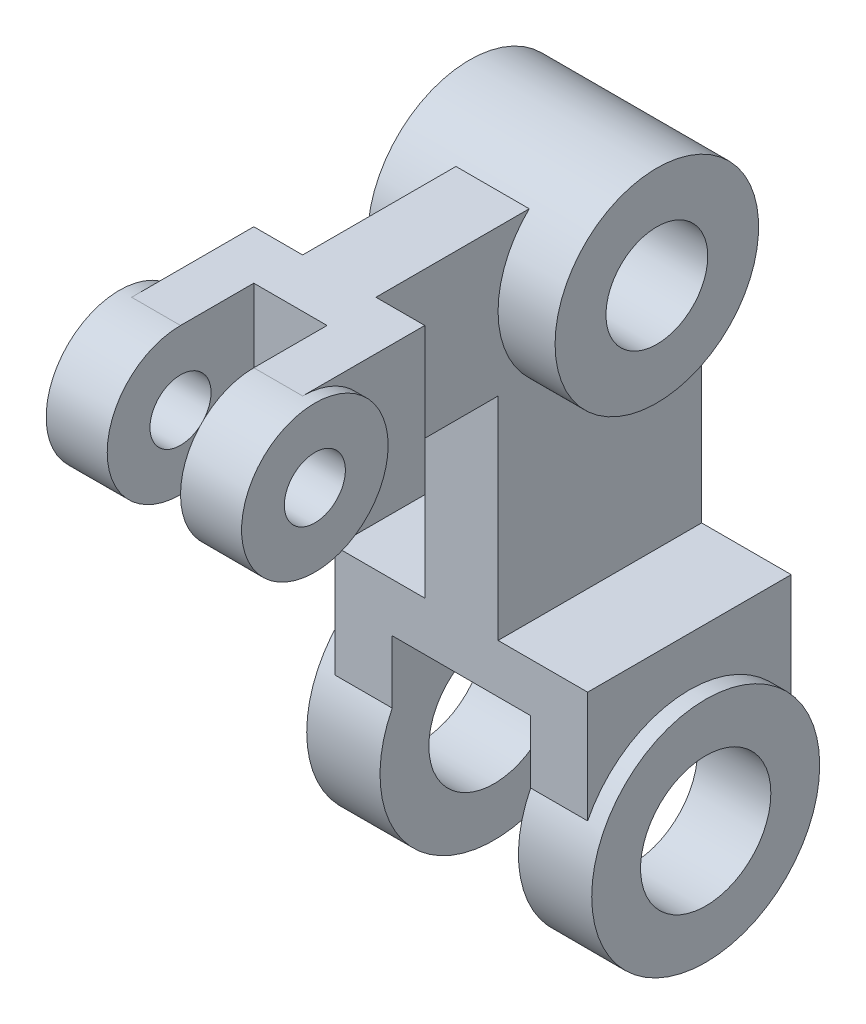
ISO-10303-21;
HEADER;
FILE_DESCRIPTION(('STEP AP214'),'2;1');
FILE_NAME('part.step','',(''),(''),'','','');
FILE_SCHEMA(('AUTOMOTIVE_DESIGN { 1 0 10303 214 1 1 1 1 }'));
ENDSEC;
DATA;
#1=APPLICATION_CONTEXT('core data for automotive mechanical design processes');
#2=APPLICATION_PROTOCOL_DEFINITION('international standard','automotive_design',2000,#1);
#3=PRODUCT_CONTEXT('',#1,'mechanical');
#4=PRODUCT('Part','Part','',(#3));
#5=PRODUCT_RELATED_PRODUCT_CATEGORY('part','',(#4));
#6=PRODUCT_DEFINITION_FORMATION('','',#4);
#7=PRODUCT_DEFINITION_CONTEXT('part definition',#1,'design');
#8=PRODUCT_DEFINITION('design','',#6,#7);
#9=PRODUCT_DEFINITION_SHAPE('','',#8);
#10=(LENGTH_UNIT() NAMED_UNIT(*) SI_UNIT(.MILLI.,.METRE.));
#11=(NAMED_UNIT(*) PLANE_ANGLE_UNIT() SI_UNIT($,.RADIAN.));
#12=(NAMED_UNIT(*) SI_UNIT($,.STERADIAN.) SOLID_ANGLE_UNIT());
#13=UNCERTAINTY_MEASURE_WITH_UNIT(LENGTH_MEASURE(1.E-05),#10,'distance_accuracy_value','');
#14=(GEOMETRIC_REPRESENTATION_CONTEXT(3) GLOBAL_UNCERTAINTY_ASSIGNED_CONTEXT((#13)) GLOBAL_UNIT_ASSIGNED_CONTEXT((#10,
#11,#12)) REPRESENTATION_CONTEXT('',''));
#15=CARTESIAN_POINT('',(0.,0.,0.));
#16=DIRECTION('',(0.,0.,1.));
#17=DIRECTION('',(1.,0.,0.));
#18=AXIS2_PLACEMENT_3D('',#15,#16,#17);
#19=CARTESIAN_POINT('',(-12.,110.,0.));
#20=DIRECTION('',(-1.,0.,0.));
#21=DIRECTION('',(0.,0.,1.));
#22=AXIS2_PLACEMENT_3D('',#19,#20,#21);
#23=CYLINDRICAL_SURFACE('',#22,25.);
#24=CARTESIAN_POINT('',(-12.,110.,0.));
#25=DIRECTION('',(-1.,0.,0.));
#26=DIRECTION('',(0.,0.,1.));
#27=AXIS2_PLACEMENT_3D('',#24,#25,#26);
#28=CIRCLE('',#27,25.);
#29=CARTESIAN_POINT('',(-12.,110.,25.));
#30=VERTEX_POINT('',#29);
#31=EDGE_CURVE('E265',#30,#30,#28,.T.);
#32=ORIENTED_EDGE('',*,*,#31,.T.);
#33=EDGE_LOOP('',(#32));
#34=FACE_BOUND('',#33,.T.);
#35=CARTESIAN_POINT('',(-58.,110.,0.));
#36=DIRECTION('',(-1.,0.,0.));
#37=DIRECTION('',(0.,0.,1.));
#38=AXIS2_PLACEMENT_3D('',#35,#36,#37);
#39=CIRCLE('',#38,25.);
#40=CARTESIAN_POINT('',(-58.,110.,25.));
#41=VERTEX_POINT('',#40);
#42=EDGE_CURVE('E258',#41,#41,#39,.T.);
#43=ORIENTED_EDGE('',*,*,#42,.F.);
#44=EDGE_LOOP('',(#43));
#45=FACE_BOUND('',#44,.T.);
#46=DIRECTION('',(-1.,0.,0.));
#47=VECTOR('',#46,1.);
#48=CARTESIAN_POINT('',(-12.,128.,17.3493515728975));
#49=LINE('',#48,#47);
#50=CARTESIAN_POINT('',(-44.,128.,17.3493515728975));
#51=VERTEX_POINT('',#50);
#52=CARTESIAN_POINT('',(-26.,128.,17.3493515728975));
#53=VERTEX_POINT('',#52);
#54=EDGE_CURVE('E11',#51,#53,#49,.F.);
#55=ORIENTED_EDGE('',*,*,#54,.T.);
#56=CARTESIAN_POINT('',(-26.,110.,0.));
#57=DIRECTION('',(1.,0.,0.));
#58=DIRECTION('',(0.,1.,0.));
#59=AXIS2_PLACEMENT_3D('',#56,#57,#58);
#60=CIRCLE('',#59,25.);
#61=CARTESIAN_POINT('',(-26.,110.,-25.));
#62=VERTEX_POINT('',#61);
#63=EDGE_CURVE('E57',#53,#62,#60,.T.);
#64=ORIENTED_EDGE('',*,*,#63,.T.);
#65=DIRECTION('',(-1.,0.,0.));
#66=VECTOR('',#65,1.);
#67=CARTESIAN_POINT('',(-44.,110.,-25.));
#68=LINE('',#67,#66);
#69=CARTESIAN_POINT('',(-44.,110.,-25.));
#70=VERTEX_POINT('',#69);
#71=EDGE_CURVE('E275',#62,#70,#68,.T.);
#72=ORIENTED_EDGE('',*,*,#71,.T.);
#73=CARTESIAN_POINT('',(-44.,110.,0.));
#74=DIRECTION('',(-1.,0.,0.));
#75=DIRECTION('',(0.,0.,1.));
#76=AXIS2_PLACEMENT_3D('',#73,#74,#75);
#77=CIRCLE('',#76,25.);
#78=EDGE_CURVE('E261',#70,#51,#77,.T.);
#79=ORIENTED_EDGE('',*,*,#78,.T.);
#80=EDGE_LOOP('',(#55,#64,#72,#79));
#81=FACE_BOUND('',#80,.T.);
#82=ADVANCED_FACE('F50',(#34,#45,#81),#23,.T.);
#83=CARTESIAN_POINT('',(0.,40.,28.));
#84=DIRECTION('',(0.,-1.,0.));
#85=DIRECTION('',(1.,0.,0.));
#86=AXIS2_PLACEMENT_3D('',#83,#84,#85);
#87=PLANE('',#86);
#88=DIRECTION('',(0.,0.,1.));
#89=VECTOR('',#88,1.);
#90=CARTESIAN_POINT('',(-44.,40.,-25.));
#91=LINE('',#90,#89);
#92=CARTESIAN_POINT('',(-44.,40.,-25.));
#93=VERTEX_POINT('',#92);
#94=CARTESIAN_POINT('',(-44.,40.,25.));
#95=VERTEX_POINT('',#94);
#96=EDGE_CURVE('E273',#93,#95,#91,.T.);
#97=ORIENTED_EDGE('',*,*,#96,.F.);
#98=DIRECTION('',(1.,0.,0.));
#99=VECTOR('',#98,1.);
#100=CARTESIAN_POINT('',(-78.,40.,-25.));
#101=LINE('',#100,#99);
#102=CARTESIAN_POINT('',(-66.,40.,-25.));
#103=VERTEX_POINT('',#102);
#104=EDGE_CURVE('E297',#103,#93,#101,.T.);
#105=ORIENTED_EDGE('',*,*,#104,.F.);
#106=DIRECTION('',(0.,0.,-1.));
#107=VECTOR('',#106,1.);
#108=CARTESIAN_POINT('',(-66.,40.,28.));
#109=LINE('',#108,#107);
#110=CARTESIAN_POINT('',(-66.,40.,25.));
#111=VERTEX_POINT('',#110);
#112=EDGE_CURVE('E347',#111,#103,#109,.T.);
#113=ORIENTED_EDGE('',*,*,#112,.F.);
#114=DIRECTION('',(1.,0.,0.));
#115=VECTOR('',#114,1.);
#116=CARTESIAN_POINT('',(-78.,40.,25.));
#117=LINE('',#116,#115);
#118=EDGE_CURVE('E289',#111,#95,#117,.T.);
#119=ORIENTED_EDGE('',*,*,#118,.T.);
#120=EDGE_LOOP('',(#97,#105,#113,#119));
#121=FACE_BOUND('',#120,.T.);
#122=ADVANCED_FACE('F476',(#121),#87,.F.);
#123=CARTESIAN_POINT('',(-70.,0.,0.));
#124=DIRECTION('',(1.,0.,0.));
#125=DIRECTION('',(0.,0.,-1.));
#126=AXIS2_PLACEMENT_3D('',#123,#124,#125);
#127=CYLINDRICAL_SURFACE('',#126,28.);
#128=DIRECTION('',(1.,0.,0.));
#129=VECTOR('',#128,1.);
#130=CARTESIAN_POINT('',(-78.,12.6095202129185,25.));
#131=LINE('',#130,#129);
#132=CARTESIAN_POINT('',(-66.,12.6095202129185,25.));
#133=VERTEX_POINT('',#132);
#134=CARTESIAN_POINT('',(-52.,12.6095202129185,25.));
#135=VERTEX_POINT('',#134);
#136=EDGE_CURVE('E295',#133,#135,#131,.T.);
#137=ORIENTED_EDGE('',*,*,#136,.F.);
#138=CARTESIAN_POINT('',(-66.,0.,0.));
#139=DIRECTION('',(1.,0.,0.));
#140=DIRECTION('',(0.,0.,-1.));
#141=AXIS2_PLACEMENT_3D('',#138,#139,#140);
#142=CIRCLE('',#141,28.);
#143=CARTESIAN_POINT('',(-66.,12.6095202129185,-25.));
#144=VERTEX_POINT('',#143);
#145=EDGE_CURVE('E333',#133,#144,#142,.F.);
#146=ORIENTED_EDGE('',*,*,#145,.T.);
#147=DIRECTION('',(1.,0.,0.));
#148=VECTOR('',#147,1.);
#149=CARTESIAN_POINT('',(-78.,12.6095202129185,-25.));
#150=LINE('',#149,#148);
#151=CARTESIAN_POINT('',(-52.,12.6095202129185,-25.));
#152=VERTEX_POINT('',#151);
#153=EDGE_CURVE('E287',#144,#152,#150,.T.);
#154=ORIENTED_EDGE('',*,*,#153,.T.);
#155=CARTESIAN_POINT('',(-52.,0.,0.));
#156=DIRECTION('',(-1.,0.,0.));
#157=DIRECTION('',(0.,0.,1.));
#158=AXIS2_PLACEMENT_3D('',#155,#156,#157);
#159=CIRCLE('',#158,28.);
#160=EDGE_CURVE('E326',#152,#135,#159,.T.);
#161=ORIENTED_EDGE('',*,*,#160,.T.);
#162=EDGE_LOOP('',(#137,#146,#154,#161));
#163=FACE_BOUND('',#162,.T.);
#164=CARTESIAN_POINT('',(-70.,0.,0.));
#165=DIRECTION('',(-1.,0.,0.));
#166=DIRECTION('',(0.,0.,1.));
#167=AXIS2_PLACEMENT_3D('',#164,#165,#166);
#168=CIRCLE('',#167,28.);
#169=CARTESIAN_POINT('',(-70.,0.,28.));
#170=VERTEX_POINT('',#169);
#171=EDGE_CURVE('E331',#170,#170,#168,.T.);
#172=ORIENTED_EDGE('',*,*,#171,.F.);
#173=EDGE_LOOP('',(#172));
#174=FACE_BOUND('',#173,.T.);
#175=ADVANCED_FACE('F487',(#163,#174),#127,.T.);
#176=CARTESIAN_POINT('',(-18.,0.,0.));
#177=DIRECTION('',(1.,0.,0.));
#178=DIRECTION('',(0.,0.,-1.));
#179=AXIS2_PLACEMENT_3D('',#176,#177,#178);
#180=CYLINDRICAL_SURFACE('',#179,28.);
#181=CARTESIAN_POINT('',(-4.,0.,0.));
#182=DIRECTION('',(1.,0.,0.));
#183=DIRECTION('',(0.,0.,-1.));
#184=AXIS2_PLACEMENT_3D('',#181,#182,#183);
#185=CIRCLE('',#184,28.);
#186=CARTESIAN_POINT('',(-4.,12.6095202129185,25.));
#187=VERTEX_POINT('',#186);
#188=CARTESIAN_POINT('',(-4.,12.6095202129185,-25.));
#189=VERTEX_POINT('',#188);
#190=EDGE_CURVE('E352',#187,#189,#185,.F.);
#191=ORIENTED_EDGE('',*,*,#190,.F.);
#192=CARTESIAN_POINT('',(-18.,12.6095202129185,25.));
#193=VERTEX_POINT('',#192);
#194=EDGE_CURVE('E286',#193,#187,#131,.T.);
#195=ORIENTED_EDGE('',*,*,#194,.F.);
#196=CARTESIAN_POINT('',(-18.,0.,0.));
#197=DIRECTION('',(1.,0.,0.));
#198=DIRECTION('',(0.,0.,-1.));
#199=AXIS2_PLACEMENT_3D('',#196,#197,#198);
#200=CIRCLE('',#199,28.);
#201=CARTESIAN_POINT('',(-18.,12.6095202129185,-25.));
#202=VERTEX_POINT('',#201);
#203=EDGE_CURVE('E365',#193,#202,#200,.T.);
#204=ORIENTED_EDGE('',*,*,#203,.T.);
#205=EDGE_CURVE('E296',#202,#189,#150,.T.);
#206=ORIENTED_EDGE('',*,*,#205,.T.);
#207=EDGE_LOOP('',(#191,#195,#204,#206));
#208=FACE_BOUND('',#207,.T.);
#209=CARTESIAN_POINT('',(0.,0.,0.));
#210=DIRECTION('',(1.,0.,0.));
#211=DIRECTION('',(0.,0.,-1.));
#212=AXIS2_PLACEMENT_3D('',#209,#210,#211);
#213=CIRCLE('',#212,28.);
#214=CARTESIAN_POINT('',(0.,0.,-28.));
#215=VERTEX_POINT('',#214);
#216=EDGE_CURVE('E363',#215,#215,#213,.T.);
#217=ORIENTED_EDGE('',*,*,#216,.F.);
#218=EDGE_LOOP('',(#217));
#219=FACE_BOUND('',#218,.T.);
#220=ADVANCED_FACE('F47',(#208,#219),#180,.T.);
#221=CARTESIAN_POINT('',(-66.,0.,28.));
#222=DIRECTION('',(1.,0.,0.));
#223=DIRECTION('',(0.,0.,-1.));
#224=AXIS2_PLACEMENT_3D('',#221,#222,#223);
#225=PLANE('',#224);
#226=ORIENTED_EDGE('',*,*,#145,.F.);
#227=DIRECTION('',(0.,1.,0.));
#228=VECTOR('',#227,1.);
#229=CARTESIAN_POINT('',(-66.,0.,25.));
#230=LINE('',#229,#228);
#231=EDGE_CURVE('E325',#133,#111,#230,.T.);
#232=ORIENTED_EDGE('',*,*,#231,.T.);
#233=ORIENTED_EDGE('',*,*,#112,.T.);
#234=DIRECTION('',(0.,-1.,0.));
#235=VECTOR('',#234,1.);
#236=CARTESIAN_POINT('',(-66.,0.,-25.));
#237=LINE('',#236,#235);
#238=EDGE_CURVE('E311',#103,#144,#237,.T.);
#239=ORIENTED_EDGE('',*,*,#238,.T.);
#240=EDGE_LOOP('',(#226,#232,#233,#239));
#241=FACE_BOUND('',#240,.T.);
#242=ADVANCED_FACE('F484',(#241),#225,.F.);
#243=CARTESIAN_POINT('',(-18.,0.,0.));
#244=DIRECTION('',(1.,0.,0.));
#245=DIRECTION('',(0.,0.,-1.));
#246=AXIS2_PLACEMENT_3D('',#243,#244,#245);
#247=PLANE('',#246);
#248=ORIENTED_EDGE('',*,*,#203,.F.);
#249=DIRECTION('',(0.,1.,0.));
#250=VECTOR('',#249,1.);
#251=CARTESIAN_POINT('',(-18.,0.,25.));
#252=LINE('',#251,#250);
#253=CARTESIAN_POINT('',(-18.,28.,25.));
#254=VERTEX_POINT('',#253);
#255=EDGE_CURVE('E318',#193,#254,#252,.T.);
#256=ORIENTED_EDGE('',*,*,#255,.T.);
#257=DIRECTION('',(0.,0.,-1.));
#258=VECTOR('',#257,1.);
#259=CARTESIAN_POINT('',(-18.,28.,28.));
#260=LINE('',#259,#258);
#261=CARTESIAN_POINT('',(-18.,28.,-25.));
#262=VERTEX_POINT('',#261);
#263=EDGE_CURVE('E338',#254,#262,#260,.T.);
#264=ORIENTED_EDGE('',*,*,#263,.T.);
#265=DIRECTION('',(0.,-1.,0.));
#266=VECTOR('',#265,1.);
#267=CARTESIAN_POINT('',(-18.,0.,-25.));
#268=LINE('',#267,#266);
#269=EDGE_CURVE('E308',#262,#202,#268,.T.);
#270=ORIENTED_EDGE('',*,*,#269,.T.);
#271=EDGE_LOOP('',(#248,#256,#264,#270));
#272=FACE_BOUND('',#271,.T.);
#273=CARTESIAN_POINT('',(-18.,0.,0.));
#274=DIRECTION('',(1.,0.,0.));
#275=DIRECTION('',(0.,0.,-1.));
#276=AXIS2_PLACEMENT_3D('',#273,#274,#275);
#277=CIRCLE('',#276,16.);
#278=CARTESIAN_POINT('',(-18.,0.,-16.));
#279=VERTEX_POINT('',#278);
#280=EDGE_CURVE('E356',#279,#279,#277,.T.);
#281=ORIENTED_EDGE('',*,*,#280,.T.);
#282=EDGE_LOOP('',(#281));
#283=FACE_BOUND('',#282,.T.);
#284=ADVANCED_FACE('F502',(#272,#283),#247,.F.);
#285=CARTESIAN_POINT('',(0.,0.,0.));
#286=DIRECTION('',(1.,0.,0.));
#287=DIRECTION('',(0.,0.,-1.));
#288=AXIS2_PLACEMENT_3D('',#285,#286,#287);
#289=PLANE('',#288);
#290=CARTESIAN_POINT('',(0.,0.,0.));
#291=DIRECTION('',(1.,0.,0.));
#292=DIRECTION('',(0.,0.,-1.));
#293=AXIS2_PLACEMENT_3D('',#290,#291,#292);
#294=CIRCLE('',#293,16.);
#295=CARTESIAN_POINT('',(0.,0.,-16.));
#296=VERTEX_POINT('',#295);
#297=EDGE_CURVE('E355',#296,#296,#294,.T.);
#298=ORIENTED_EDGE('',*,*,#297,.F.);
#299=EDGE_LOOP('',(#298));
#300=FACE_BOUND('',#299,.T.);
#301=ORIENTED_EDGE('',*,*,#216,.T.);
#302=EDGE_LOOP('',(#301));
#303=FACE_BOUND('',#302,.T.);
#304=ADVANCED_FACE('F520',(#300,#303),#289,.T.);
#305=CARTESIAN_POINT('',(-95.,0.,0.));
#306=DIRECTION('',(1.,0.,0.));
#307=DIRECTION('',(0.,0.,-1.));
#308=AXIS2_PLACEMENT_3D('',#305,#306,#307);
#309=CYLINDRICAL_SURFACE('',#308,16.);
#310=ORIENTED_EDGE('',*,*,#280,.F.);
#311=EDGE_LOOP('',(#310));
#312=FACE_BOUND('',#311,.T.);
#313=ORIENTED_EDGE('',*,*,#297,.T.);
#314=EDGE_LOOP('',(#313));
#315=FACE_BOUND('',#314,.T.);
#316=ADVANCED_FACE('F517',(#312,#315),#309,.F.);
#317=CARTESIAN_POINT('',(-4.,0.,28.));
#318=DIRECTION('',(1.,0.,0.));
#319=DIRECTION('',(0.,0.,-1.));
#320=AXIS2_PLACEMENT_3D('',#317,#318,#319);
#321=PLANE('',#320);
#322=DIRECTION('',(0.,1.,0.));
#323=VECTOR('',#322,1.);
#324=CARTESIAN_POINT('',(-4.,0.,25.));
#325=LINE('',#324,#323);
#326=CARTESIAN_POINT('',(-4.,40.,25.));
#327=VERTEX_POINT('',#326);
#328=EDGE_CURVE('E283',#187,#327,#325,.T.);
#329=ORIENTED_EDGE('',*,*,#328,.F.);
#330=ORIENTED_EDGE('',*,*,#190,.T.);
#331=DIRECTION('',(0.,-1.,0.));
#332=VECTOR('',#331,1.);
#333=CARTESIAN_POINT('',(-4.,0.,-25.));
#334=LINE('',#333,#332);
#335=CARTESIAN_POINT('',(-4.,40.,-25.));
#336=VERTEX_POINT('',#335);
#337=EDGE_CURVE('E277',#336,#189,#334,.T.);
#338=ORIENTED_EDGE('',*,*,#337,.F.);
#339=DIRECTION('',(0.,0.,-1.));
#340=VECTOR('',#339,1.);
#341=CARTESIAN_POINT('',(-4.,40.,28.));
#342=LINE('',#341,#340);
#343=EDGE_CURVE('E349',#327,#336,#342,.T.);
#344=ORIENTED_EDGE('',*,*,#343,.F.);
#345=EDGE_LOOP('',(#329,#330,#338,#344));
#346=FACE_BOUND('',#345,.T.);
#347=ADVANCED_FACE('F499',(#346),#321,.T.);
#348=CARTESIAN_POINT('',(-26.,40.,-25.));
#349=VERTEX_POINT('',#348);
#350=EDGE_CURVE('E300',#349,#336,#101,.T.);
#351=ORIENTED_EDGE('',*,*,#350,.F.);
#352=DIRECTION('',(0.,0.,1.));
#353=VECTOR('',#352,1.);
#354=CARTESIAN_POINT('',(-26.,40.,-25.));
#355=LINE('',#354,#353);
#356=CARTESIAN_POINT('',(-26.,40.,25.));
#357=VERTEX_POINT('',#356);
#358=EDGE_CURVE('E280',#349,#357,#355,.T.);
#359=ORIENTED_EDGE('',*,*,#358,.T.);
#360=EDGE_CURVE('E292',#357,#327,#117,.T.);
#361=ORIENTED_EDGE('',*,*,#360,.T.);
#362=ORIENTED_EDGE('',*,*,#343,.T.);
#363=EDGE_LOOP('',(#351,#359,#361,#362));
#364=FACE_BOUND('',#363,.T.);
#365=ADVANCED_FACE('F495',(#364),#87,.F.);
#366=CARTESIAN_POINT('',(-52.,0.,28.));
#367=DIRECTION('',(-1.,0.,0.));
#368=DIRECTION('',(0.,0.,1.));
#369=AXIS2_PLACEMENT_3D('',#366,#367,#368);
#370=PLANE('',#369);
#371=DIRECTION('',(0.,-1.,0.));
#372=VECTOR('',#371,1.);
#373=CARTESIAN_POINT('',(-52.,0.,25.));
#374=LINE('',#373,#372);
#375=CARTESIAN_POINT('',(-52.,28.,25.));
#376=VERTEX_POINT('',#375);
#377=EDGE_CURVE('E320',#376,#135,#374,.T.);
#378=ORIENTED_EDGE('',*,*,#377,.T.);
#379=ORIENTED_EDGE('',*,*,#160,.F.);
#380=DIRECTION('',(0.,1.,0.));
#381=VECTOR('',#380,1.);
#382=CARTESIAN_POINT('',(-52.,0.,-25.));
#383=LINE('',#382,#381);
#384=CARTESIAN_POINT('',(-52.,28.,-25.));
#385=VERTEX_POINT('',#384);
#386=EDGE_CURVE('E304',#152,#385,#383,.T.);
#387=ORIENTED_EDGE('',*,*,#386,.T.);
#388=DIRECTION('',(0.,0.,-1.));
#389=VECTOR('',#388,1.);
#390=CARTESIAN_POINT('',(-52.,28.,28.));
#391=LINE('',#390,#389);
#392=EDGE_CURVE('E345',#376,#385,#391,.T.);
#393=ORIENTED_EDGE('',*,*,#392,.F.);
#394=EDGE_LOOP('',(#378,#379,#387,#393));
#395=FACE_BOUND('',#394,.T.);
#396=CARTESIAN_POINT('',(-52.,0.,0.));
#397=DIRECTION('',(-1.,0.,0.));
#398=DIRECTION('',(0.,0.,1.));
#399=AXIS2_PLACEMENT_3D('',#396,#397,#398);
#400=CIRCLE('',#399,16.);
#401=CARTESIAN_POINT('',(-52.,0.,16.));
#402=VERTEX_POINT('',#401);
#403=EDGE_CURVE('E327',#402,#402,#400,.T.);
#404=ORIENTED_EDGE('',*,*,#403,.T.);
#405=EDGE_LOOP('',(#404));
#406=FACE_BOUND('',#405,.T.);
#407=ADVANCED_FACE('F515',(#395,#406),#370,.F.);
#408=CARTESIAN_POINT('',(0.,28.,28.));
#409=DIRECTION('',(0.,1.,0.));
#410=DIRECTION('',(0.,0.,1.));
#411=AXIS2_PLACEMENT_3D('',#408,#409,#410);
#412=PLANE('',#411);
#413=ORIENTED_EDGE('',*,*,#263,.F.);
#414=DIRECTION('',(-1.,0.,0.));
#415=VECTOR('',#414,1.);
#416=CARTESIAN_POINT('',(0.,28.,25.));
#417=LINE('',#416,#415);
#418=EDGE_CURVE('E313',#254,#376,#417,.T.);
#419=ORIENTED_EDGE('',*,*,#418,.T.);
#420=ORIENTED_EDGE('',*,*,#392,.T.);
#421=DIRECTION('',(1.,0.,0.));
#422=VECTOR('',#421,1.);
#423=CARTESIAN_POINT('',(0.,28.,-25.));
#424=LINE('',#423,#422);
#425=EDGE_CURVE('E293',#385,#262,#424,.T.);
#426=ORIENTED_EDGE('',*,*,#425,.T.);
#427=EDGE_LOOP('',(#413,#419,#420,#426));
#428=FACE_BOUND('',#427,.T.);
#429=ADVANCED_FACE('F507',(#428),#412,.F.);
#430=CARTESIAN_POINT('',(-70.,0.,0.));
#431=DIRECTION('',(-1.,0.,0.));
#432=DIRECTION('',(0.,0.,1.));
#433=AXIS2_PLACEMENT_3D('',#430,#431,#432);
#434=PLANE('',#433);
#435=CARTESIAN_POINT('',(-70.,0.,0.));
#436=DIRECTION('',(-1.,0.,0.));
#437=DIRECTION('',(0.,0.,1.));
#438=AXIS2_PLACEMENT_3D('',#435,#436,#437);
#439=CIRCLE('',#438,16.);
#440=CARTESIAN_POINT('',(-70.,0.,16.));
#441=VERTEX_POINT('',#440);
#442=EDGE_CURVE('E330',#441,#441,#439,.T.);
#443=ORIENTED_EDGE('',*,*,#442,.F.);
#444=EDGE_LOOP('',(#443));
#445=FACE_BOUND('',#444,.T.);
#446=ORIENTED_EDGE('',*,*,#171,.T.);
#447=EDGE_LOOP('',(#446));
#448=FACE_BOUND('',#447,.T.);
#449=ADVANCED_FACE('F551',(#445,#448),#434,.T.);
#450=CARTESIAN_POINT('',(-95.,0.,0.));
#451=DIRECTION('',(1.,0.,0.));
#452=DIRECTION('',(0.,0.,-1.));
#453=AXIS2_PLACEMENT_3D('',#450,#451,#452);
#454=CYLINDRICAL_SURFACE('',#453,16.);
#455=ORIENTED_EDGE('',*,*,#403,.F.);
#456=EDGE_LOOP('',(#455));
#457=FACE_BOUND('',#456,.T.);
#458=ORIENTED_EDGE('',*,*,#442,.T.);
#459=EDGE_LOOP('',(#458));
#460=FACE_BOUND('',#459,.T.);
#461=ADVANCED_FACE('F550',(#457,#460),#454,.F.);
#462=CARTESIAN_POINT('',(-78.,0.,-25.));
#463=DIRECTION('',(0.,0.,1.));
#464=DIRECTION('',(0.,-1.,0.));
#465=AXIS2_PLACEMENT_3D('',#462,#463,#464);
#466=PLANE('',#465);
#467=ORIENTED_EDGE('',*,*,#104,.T.);
#468=DIRECTION('',(0.,-1.,0.));
#469=VECTOR('',#468,1.);
#470=CARTESIAN_POINT('',(-44.,40.,-25.));
#471=LINE('',#470,#469);
#472=EDGE_CURVE('E269',#70,#93,#471,.T.);
#473=ORIENTED_EDGE('',*,*,#472,.F.);
#474=ORIENTED_EDGE('',*,*,#71,.F.);
#475=DIRECTION('',(0.,1.,0.));
#476=VECTOR('',#475,1.);
#477=CARTESIAN_POINT('',(-26.,110.,-25.));
#478=LINE('',#477,#476);
#479=EDGE_CURVE('E270',#349,#62,#478,.T.);
#480=ORIENTED_EDGE('',*,*,#479,.F.);
#481=ORIENTED_EDGE('',*,*,#350,.T.);
#482=ORIENTED_EDGE('',*,*,#337,.T.);
#483=ORIENTED_EDGE('',*,*,#205,.F.);
#484=ORIENTED_EDGE('',*,*,#269,.F.);
#485=ORIENTED_EDGE('',*,*,#425,.F.);
#486=ORIENTED_EDGE('',*,*,#386,.F.);
#487=ORIENTED_EDGE('',*,*,#153,.F.);
#488=ORIENTED_EDGE('',*,*,#238,.F.);
#489=EDGE_LOOP('',(#467,#473,#474,#480,#481,#482,#483,#484,#485,#486,#487,#488));
#490=FACE_BOUND('',#489,.T.);
#491=ADVANCED_FACE('F472',(#490),#466,.F.);
#492=CARTESIAN_POINT('',(-78.,0.,25.));
#493=DIRECTION('',(0.,0.,-1.));
#494=DIRECTION('',(-1.,0.,0.));
#495=AXIS2_PLACEMENT_3D('',#492,#493,#494);
#496=PLANE('',#495);
#497=DIRECTION('',(0.,1.,0.));
#498=VECTOR('',#497,1.);
#499=CARTESIAN_POINT('',(-26.,110.,25.));
#500=LINE('',#499,#498);
#501=CARTESIAN_POINT('',(-26.,92.,25.));
#502=VERTEX_POINT('',#501);
#503=EDGE_CURVE('E66',#357,#502,#500,.T.);
#504=ORIENTED_EDGE('',*,*,#503,.T.);
#505=DIRECTION('',(-1.,0.,0.));
#506=VECTOR('',#505,1.);
#507=CARTESIAN_POINT('',(-78.,92.,25.));
#508=LINE('',#507,#506);
#509=CARTESIAN_POINT('',(-44.,92.,25.));
#510=VERTEX_POINT('',#509);
#511=EDGE_CURVE('E259',#502,#510,#508,.T.);
#512=ORIENTED_EDGE('',*,*,#511,.T.);
#513=DIRECTION('',(0.,-1.,0.));
#514=VECTOR('',#513,1.);
#515=CARTESIAN_POINT('',(-44.,40.,25.));
#516=LINE('',#515,#514);
#517=EDGE_CURVE('E267',#510,#95,#516,.T.);
#518=ORIENTED_EDGE('',*,*,#517,.T.);
#519=ORIENTED_EDGE('',*,*,#118,.F.);
#520=ORIENTED_EDGE('',*,*,#231,.F.);
#521=ORIENTED_EDGE('',*,*,#136,.T.);
#522=ORIENTED_EDGE('',*,*,#377,.F.);
#523=ORIENTED_EDGE('',*,*,#418,.F.);
#524=ORIENTED_EDGE('',*,*,#255,.F.);
#525=ORIENTED_EDGE('',*,*,#194,.T.);
#526=ORIENTED_EDGE('',*,*,#328,.T.);
#527=ORIENTED_EDGE('',*,*,#360,.F.);
#528=EDGE_LOOP('',(#504,#512,#518,#519,#520,#521,#522,#523,#524,#525,#526,#527));
#529=FACE_BOUND('',#528,.T.);
#530=ADVANCED_FACE('F442',(#529),#496,.F.);
#531=CARTESIAN_POINT('',(-44.,40.,-25.));
#532=DIRECTION('',(-1.,0.,0.));
#533=DIRECTION('',(0.,0.,1.));
#534=AXIS2_PLACEMENT_3D('',#531,#532,#533);
#535=PLANE('',#534);
#536=ORIENTED_EDGE('',*,*,#517,.F.);
#537=DIRECTION('',(0.,0.,1.));
#538=VECTOR('',#537,1.);
#539=CARTESIAN_POINT('',(-44.,92.,55.));
#540=LINE('',#539,#538);
#541=CARTESIAN_POINT('',(-44.,92.,55.));
#542=VERTEX_POINT('',#541);
#543=EDGE_CURVE('E424',#510,#542,#540,.T.);
#544=ORIENTED_EDGE('',*,*,#543,.T.);
#545=DIRECTION('',(0.,-1.,0.));
#546=VECTOR('',#545,1.);
#547=CARTESIAN_POINT('',(-44.,128.,55.));
#548=LINE('',#547,#546);
#549=CARTESIAN_POINT('',(-44.,128.,55.));
#550=VERTEX_POINT('',#549);
#551=EDGE_CURVE('E250',#550,#542,#548,.T.);
#552=ORIENTED_EDGE('',*,*,#551,.F.);
#553=DIRECTION('',(0.,0.,1.));
#554=VECTOR('',#553,1.);
#555=CARTESIAN_POINT('',(-44.,128.,55.));
#556=LINE('',#555,#554);
#557=EDGE_CURVE('E404',#51,#550,#556,.T.);
#558=ORIENTED_EDGE('',*,*,#557,.F.);
#559=ORIENTED_EDGE('',*,*,#78,.F.);
#560=ORIENTED_EDGE('',*,*,#472,.T.);
#561=ORIENTED_EDGE('',*,*,#96,.T.);
#562=EDGE_LOOP('',(#536,#544,#552,#558,#559,#560,#561));
#563=FACE_BOUND('',#562,.T.);
#564=ADVANCED_FACE('F439',(#563),#535,.T.);
#565=CARTESIAN_POINT('',(-26.,110.,-25.));
#566=DIRECTION('',(1.,0.,0.));
#567=DIRECTION('',(0.,1.,0.));
#568=AXIS2_PLACEMENT_3D('',#565,#566,#567);
#569=PLANE('',#568);
#570=ORIENTED_EDGE('',*,*,#479,.T.);
#571=ORIENTED_EDGE('',*,*,#63,.F.);
#572=DIRECTION('',(0.,0.,-1.));
#573=VECTOR('',#572,1.);
#574=CARTESIAN_POINT('',(-26.,128.,0.));
#575=LINE('',#574,#573);
#576=CARTESIAN_POINT('',(-26.,128.,55.));
#577=VERTEX_POINT('',#576);
#578=EDGE_CURVE('E405',#577,#53,#575,.T.);
#579=ORIENTED_EDGE('',*,*,#578,.F.);
#580=DIRECTION('',(0.,-1.,0.));
#581=VECTOR('',#580,1.);
#582=CARTESIAN_POINT('',(-26.,128.,55.));
#583=LINE('',#582,#581);
#584=CARTESIAN_POINT('',(-26.,92.,55.));
#585=VERTEX_POINT('',#584);
#586=EDGE_CURVE('E249',#577,#585,#583,.T.);
#587=ORIENTED_EDGE('',*,*,#586,.T.);
#588=DIRECTION('',(0.,0.,-1.));
#589=VECTOR('',#588,1.);
#590=CARTESIAN_POINT('',(-26.,92.,0.));
#591=LINE('',#590,#589);
#592=EDGE_CURVE('E421',#585,#502,#591,.T.);
#593=ORIENTED_EDGE('',*,*,#592,.T.);
#594=ORIENTED_EDGE('',*,*,#503,.F.);
#595=ORIENTED_EDGE('',*,*,#358,.F.);
#596=EDGE_LOOP('',(#570,#571,#579,#587,#593,#594,#595));
#597=FACE_BOUND('',#596,.T.);
#598=ADVANCED_FACE('F450',(#597),#569,.T.);
#599=CARTESIAN_POINT('',(-12.,110.,0.));
#600=DIRECTION('',(-1.,0.,0.));
#601=DIRECTION('',(0.,0.,1.));
#602=AXIS2_PLACEMENT_3D('',#599,#600,#601);
#603=PLANE('',#602);
#604=CARTESIAN_POINT('',(-12.,110.,0.));
#605=DIRECTION('',(1.,0.,0.));
#606=DIRECTION('',(0.,0.,-1.));
#607=AXIS2_PLACEMENT_3D('',#604,#605,#606);
#608=CIRCLE('',#607,12.5);
#609=CARTESIAN_POINT('',(-12.,110.,-12.5));
#610=VERTEX_POINT('',#609);
#611=EDGE_CURVE('E378',#610,#610,#608,.T.);
#612=ORIENTED_EDGE('',*,*,#611,.F.);
#613=EDGE_LOOP('',(#612));
#614=FACE_BOUND('',#613,.T.);
#615=ORIENTED_EDGE('',*,*,#31,.F.);
#616=EDGE_LOOP('',(#615));
#617=FACE_BOUND('',#616,.T.);
#618=ADVANCED_FACE('F537',(#614,#617),#603,.F.);
#619=CARTESIAN_POINT('',(-58.,110.,0.));
#620=DIRECTION('',(-1.,0.,0.));
#621=DIRECTION('',(0.,0.,1.));
#622=AXIS2_PLACEMENT_3D('',#619,#620,#621);
#623=PLANE('',#622);
#624=CARTESIAN_POINT('',(-58.,110.,0.));
#625=DIRECTION('',(-1.,0.,0.));
#626=DIRECTION('',(0.,0.,1.));
#627=AXIS2_PLACEMENT_3D('',#624,#625,#626);
#628=CIRCLE('',#627,12.5);
#629=CARTESIAN_POINT('',(-58.,110.,12.5));
#630=VERTEX_POINT('',#629);
#631=EDGE_CURVE('E51',#630,#630,#628,.T.);
#632=ORIENTED_EDGE('',*,*,#631,.F.);
#633=EDGE_LOOP('',(#632));
#634=FACE_BOUND('',#633,.T.);
#635=ORIENTED_EDGE('',*,*,#42,.T.);
#636=EDGE_LOOP('',(#635));
#637=FACE_BOUND('',#636,.T.);
#638=ADVANCED_FACE('F606',(#634,#637),#623,.T.);
#639=CARTESIAN_POINT('',(0.,92.,0.));
#640=DIRECTION('',(0.,-1.,0.));
#641=DIRECTION('',(0.,0.,-1.));
#642=AXIS2_PLACEMENT_3D('',#639,#640,#641);
#643=PLANE('',#642);
#644=ORIENTED_EDGE('',*,*,#511,.F.);
#645=ORIENTED_EDGE('',*,*,#592,.F.);
#646=DIRECTION('',(-1.,0.,0.));
#647=VECTOR('',#646,1.);
#648=CARTESIAN_POINT('',(-26.,92.,55.));
#649=LINE('',#648,#647);
#650=CARTESIAN_POINT('',(-14.,92.,55.));
#651=VERTEX_POINT('',#650);
#652=EDGE_CURVE('E423',#651,#585,#649,.T.);
#653=ORIENTED_EDGE('',*,*,#652,.F.);
#654=DIRECTION('',(0.,0.,-1.));
#655=VECTOR('',#654,1.);
#656=CARTESIAN_POINT('',(-14.,92.,55.));
#657=LINE('',#656,#655);
#658=CARTESIAN_POINT('',(-14.,92.,85.));
#659=VERTEX_POINT('',#658);
#660=EDGE_CURVE('E418',#659,#651,#657,.T.);
#661=ORIENTED_EDGE('',*,*,#660,.F.);
#662=DIRECTION('',(1.,0.,0.));
#663=VECTOR('',#662,1.);
#664=CARTESIAN_POINT('',(-14.,92.,85.));
#665=LINE('',#664,#663);
#666=CARTESIAN_POINT('',(-26.,92.,85.));
#667=VERTEX_POINT('',#666);
#668=EDGE_CURVE('E391',#667,#659,#665,.T.);
#669=ORIENTED_EDGE('',*,*,#668,.F.);
#670=DIRECTION('',(0.,0.,1.));
#671=VECTOR('',#670,1.);
#672=CARTESIAN_POINT('',(-26.,92.,85.));
#673=LINE('',#672,#671);
#674=CARTESIAN_POINT('',(-26.,92.,67.));
#675=VERTEX_POINT('',#674);
#676=EDGE_CURVE('E235',#675,#667,#673,.T.);
#677=ORIENTED_EDGE('',*,*,#676,.F.);
#678=DIRECTION('',(1.,0.,0.));
#679=VECTOR('',#678,1.);
#680=CARTESIAN_POINT('',(-26.,92.,67.));
#681=LINE('',#680,#679);
#682=CARTESIAN_POINT('',(-44.,92.,67.));
#683=VERTEX_POINT('',#682);
#684=EDGE_CURVE('E229',#683,#675,#681,.T.);
#685=ORIENTED_EDGE('',*,*,#684,.F.);
#686=DIRECTION('',(0.,0.,-1.));
#687=VECTOR('',#686,1.);
#688=CARTESIAN_POINT('',(-44.,92.,67.));
#689=LINE('',#688,#687);
#690=CARTESIAN_POINT('',(-44.,92.,85.));
#691=VERTEX_POINT('',#690);
#692=EDGE_CURVE('E213',#691,#683,#689,.T.);
#693=ORIENTED_EDGE('',*,*,#692,.F.);
#694=DIRECTION('',(1.,0.,0.));
#695=VECTOR('',#694,1.);
#696=CARTESIAN_POINT('',(-44.,92.,85.));
#697=LINE('',#696,#695);
#698=CARTESIAN_POINT('',(-56.,92.,85.));
#699=VERTEX_POINT('',#698);
#700=EDGE_CURVE('E204',#699,#691,#697,.T.);
#701=ORIENTED_EDGE('',*,*,#700,.F.);
#702=DIRECTION('',(0.,0.,1.));
#703=VECTOR('',#702,1.);
#704=CARTESIAN_POINT('',(-56.,92.,85.));
#705=LINE('',#704,#703);
#706=CARTESIAN_POINT('',(-56.,92.,55.));
#707=VERTEX_POINT('',#706);
#708=EDGE_CURVE('E212',#707,#699,#705,.T.);
#709=ORIENTED_EDGE('',*,*,#708,.F.);
#710=DIRECTION('',(-1.,0.,0.));
#711=VECTOR('',#710,1.);
#712=CARTESIAN_POINT('',(-56.,92.,55.));
#713=LINE('',#712,#711);
#714=EDGE_CURVE('E430',#542,#707,#713,.T.);
#715=ORIENTED_EDGE('',*,*,#714,.F.);
#716=ORIENTED_EDGE('',*,*,#543,.F.);
#717=EDGE_LOOP('',(#644,#645,#653,#661,#669,#677,#685,#693,#701,#709,#715,#716));
#718=FACE_BOUND('',#717,.T.);
#719=ADVANCED_FACE('F227',(#718),#643,.T.);
#720=CARTESIAN_POINT('',(-14.,128.,55.));
#721=DIRECTION('',(-1.,0.,0.));
#722=DIRECTION('',(0.,0.,1.));
#723=AXIS2_PLACEMENT_3D('',#720,#721,#722);
#724=PLANE('',#723);
#725=DIRECTION('',(0.,0.,-1.));
#726=VECTOR('',#725,1.);
#727=CARTESIAN_POINT('',(-14.,128.,55.));
#728=LINE('',#727,#726);
#729=CARTESIAN_POINT('',(-14.,128.,85.));
#730=VERTEX_POINT('',#729);
#731=CARTESIAN_POINT('',(-14.,128.,55.));
#732=VERTEX_POINT('',#731);
#733=EDGE_CURVE('E399',#730,#732,#728,.T.);
#734=ORIENTED_EDGE('',*,*,#733,.F.);
#735=CARTESIAN_POINT('',(-14.,110.,85.));
#736=DIRECTION('',(-1.,0.,0.));
#737=DIRECTION('',(0.,0.,1.));
#738=AXIS2_PLACEMENT_3D('',#735,#736,#737);
#739=CIRCLE('',#738,18.);
#740=EDGE_CURVE('E395',#730,#659,#739,.T.);
#741=ORIENTED_EDGE('',*,*,#740,.T.);
#742=ORIENTED_EDGE('',*,*,#660,.T.);
#743=DIRECTION('',(0.,-1.,0.));
#744=VECTOR('',#743,1.);
#745=CARTESIAN_POINT('',(-14.,128.,55.));
#746=LINE('',#745,#744);
#747=EDGE_CURVE('E254',#732,#651,#746,.T.);
#748=ORIENTED_EDGE('',*,*,#747,.F.);
#749=EDGE_LOOP('',(#734,#741,#742,#748));
#750=FACE_BOUND('',#749,.T.);
#751=ADVANCED_FACE('F460',(#750),#724,.F.);
#752=CARTESIAN_POINT('',(-26.,128.,55.));
#753=DIRECTION('',(0.,0.,1.));
#754=DIRECTION('',(1.,0.,0.));
#755=AXIS2_PLACEMENT_3D('',#752,#753,#754);
#756=PLANE('',#755);
#757=ORIENTED_EDGE('',*,*,#652,.T.);
#758=ORIENTED_EDGE('',*,*,#586,.F.);
#759=DIRECTION('',(-1.,0.,0.));
#760=VECTOR('',#759,1.);
#761=CARTESIAN_POINT('',(-26.,128.,55.));
#762=LINE('',#761,#760);
#763=EDGE_CURVE('E400',#732,#577,#762,.T.);
#764=ORIENTED_EDGE('',*,*,#763,.F.);
#765=ORIENTED_EDGE('',*,*,#747,.T.);
#766=EDGE_LOOP('',(#757,#758,#764,#765));
#767=FACE_BOUND('',#766,.T.);
#768=ADVANCED_FACE('F454',(#767),#756,.F.);
#769=CARTESIAN_POINT('',(-56.,128.,55.));
#770=DIRECTION('',(0.,0.,1.));
#771=DIRECTION('',(1.,0.,0.));
#772=AXIS2_PLACEMENT_3D('',#769,#770,#771);
#773=PLANE('',#772);
#774=ORIENTED_EDGE('',*,*,#714,.T.);
#775=DIRECTION('',(0.,-1.,0.));
#776=VECTOR('',#775,1.);
#777=CARTESIAN_POINT('',(-56.,128.,55.));
#778=LINE('',#777,#776);
#779=CARTESIAN_POINT('',(-56.,128.,55.));
#780=VERTEX_POINT('',#779);
#781=EDGE_CURVE('E242',#780,#707,#778,.T.);
#782=ORIENTED_EDGE('',*,*,#781,.F.);
#783=DIRECTION('',(-1.,0.,0.));
#784=VECTOR('',#783,1.);
#785=CARTESIAN_POINT('',(-56.,128.,55.));
#786=LINE('',#785,#784);
#787=EDGE_CURVE('E409',#550,#780,#786,.T.);
#788=ORIENTED_EDGE('',*,*,#787,.F.);
#789=ORIENTED_EDGE('',*,*,#551,.T.);
#790=EDGE_LOOP('',(#774,#782,#788,#789));
#791=FACE_BOUND('',#790,.T.);
#792=ADVANCED_FACE('F432',(#791),#773,.F.);
#793=CARTESIAN_POINT('',(-56.,128.,85.));
#794=DIRECTION('',(1.,0.,0.));
#795=DIRECTION('',(0.,0.,-1.));
#796=AXIS2_PLACEMENT_3D('',#793,#794,#795);
#797=PLANE('',#796);
#798=ORIENTED_EDGE('',*,*,#708,.T.);
#799=CARTESIAN_POINT('',(-56.,110.,85.));
#800=DIRECTION('',(1.,0.,0.));
#801=DIRECTION('',(0.,0.,-1.));
#802=AXIS2_PLACEMENT_3D('',#799,#800,#801);
#803=CIRCLE('',#802,18.);
#804=CARTESIAN_POINT('',(-56.,128.,85.));
#805=VERTEX_POINT('',#804);
#806=EDGE_CURVE('E209',#699,#805,#803,.T.);
#807=ORIENTED_EDGE('',*,*,#806,.T.);
#808=DIRECTION('',(0.,0.,1.));
#809=VECTOR('',#808,1.);
#810=CARTESIAN_POINT('',(-56.,128.,85.));
#811=LINE('',#810,#809);
#812=EDGE_CURVE('E410',#780,#805,#811,.T.);
#813=ORIENTED_EDGE('',*,*,#812,.F.);
#814=ORIENTED_EDGE('',*,*,#781,.T.);
#815=EDGE_LOOP('',(#798,#807,#813,#814));
#816=FACE_BOUND('',#815,.T.);
#817=ADVANCED_FACE('F429',(#816),#797,.F.);
#818=CARTESIAN_POINT('',(-44.,128.,67.));
#819=DIRECTION('',(-1.,0.,0.));
#820=DIRECTION('',(0.,0.,1.));
#821=AXIS2_PLACEMENT_3D('',#818,#819,#820);
#822=PLANE('',#821);
#823=CARTESIAN_POINT('',(-44.,110.,85.));
#824=DIRECTION('',(-1.,0.,0.));
#825=DIRECTION('',(0.,0.,1.));
#826=AXIS2_PLACEMENT_3D('',#823,#824,#825);
#827=CIRCLE('',#826,7.50000000000001);
#828=CARTESIAN_POINT('',(-44.,110.,92.5));
#829=VERTEX_POINT('',#828);
#830=EDGE_CURVE('E225',#829,#829,#827,.T.);
#831=ORIENTED_EDGE('',*,*,#830,.T.);
#832=EDGE_LOOP('',(#831));
#833=FACE_BOUND('',#832,.T.);
#834=ORIENTED_EDGE('',*,*,#692,.T.);
#835=DIRECTION('',(0.,-1.,0.));
#836=VECTOR('',#835,1.);
#837=CARTESIAN_POINT('',(-44.,128.,67.));
#838=LINE('',#837,#836);
#839=CARTESIAN_POINT('',(-44.,128.,67.));
#840=VERTEX_POINT('',#839);
#841=EDGE_CURVE('E241',#840,#683,#838,.T.);
#842=ORIENTED_EDGE('',*,*,#841,.F.);
#843=DIRECTION('',(0.,0.,-1.));
#844=VECTOR('',#843,1.);
#845=CARTESIAN_POINT('',(-44.,128.,67.));
#846=LINE('',#845,#844);
#847=CARTESIAN_POINT('',(-44.,128.,85.));
#848=VERTEX_POINT('',#847);
#849=EDGE_CURVE('E224',#848,#840,#846,.T.);
#850=ORIENTED_EDGE('',*,*,#849,.F.);
#851=CARTESIAN_POINT('',(-44.,110.,85.));
#852=DIRECTION('',(1.,0.,0.));
#853=DIRECTION('',(0.,0.,-1.));
#854=AXIS2_PLACEMENT_3D('',#851,#852,#853);
#855=CIRCLE('',#854,18.);
#856=EDGE_CURVE('E207',#848,#691,#855,.T.);
#857=ORIENTED_EDGE('',*,*,#856,.T.);
#858=EDGE_LOOP('',(#834,#842,#850,#857));
#859=FACE_BOUND('',#858,.T.);
#860=ADVANCED_FACE('F216',(#833,#859),#822,.F.);
#861=CARTESIAN_POINT('',(-26.,128.,67.));
#862=DIRECTION('',(0.,0.,-1.));
#863=DIRECTION('',(-1.,0.,0.));
#864=AXIS2_PLACEMENT_3D('',#861,#862,#863);
#865=PLANE('',#864);
#866=ORIENTED_EDGE('',*,*,#684,.T.);
#867=DIRECTION('',(0.,-1.,0.));
#868=VECTOR('',#867,1.);
#869=CARTESIAN_POINT('',(-26.,128.,67.));
#870=LINE('',#869,#868);
#871=CARTESIAN_POINT('',(-26.,128.,67.));
#872=VERTEX_POINT('',#871);
#873=EDGE_CURVE('E237',#872,#675,#870,.T.);
#874=ORIENTED_EDGE('',*,*,#873,.F.);
#875=DIRECTION('',(1.,0.,0.));
#876=VECTOR('',#875,1.);
#877=CARTESIAN_POINT('',(-26.,128.,67.));
#878=LINE('',#877,#876);
#879=EDGE_CURVE('E414',#840,#872,#878,.T.);
#880=ORIENTED_EDGE('',*,*,#879,.F.);
#881=ORIENTED_EDGE('',*,*,#841,.T.);
#882=EDGE_LOOP('',(#866,#874,#880,#881));
#883=FACE_BOUND('',#882,.T.);
#884=ADVANCED_FACE('F470',(#883),#865,.F.);
#885=CARTESIAN_POINT('',(-26.,128.,85.));
#886=DIRECTION('',(1.,0.,0.));
#887=DIRECTION('',(0.,0.,-1.));
#888=AXIS2_PLACEMENT_3D('',#885,#886,#887);
#889=PLANE('',#888);
#890=CARTESIAN_POINT('',(-26.,110.,85.));
#891=DIRECTION('',(1.,0.,0.));
#892=DIRECTION('',(0.,0.,-1.));
#893=AXIS2_PLACEMENT_3D('',#890,#891,#892);
#894=CIRCLE('',#893,7.50000000000001);
#895=CARTESIAN_POINT('',(-26.,110.,77.5));
#896=VERTEX_POINT('',#895);
#897=EDGE_CURVE('E368',#896,#896,#894,.T.);
#898=ORIENTED_EDGE('',*,*,#897,.T.);
#899=EDGE_LOOP('',(#898));
#900=FACE_BOUND('',#899,.T.);
#901=ORIENTED_EDGE('',*,*,#676,.T.);
#902=CARTESIAN_POINT('',(-26.,110.,85.));
#903=DIRECTION('',(1.,0.,0.));
#904=DIRECTION('',(0.,0.,-1.));
#905=AXIS2_PLACEMENT_3D('',#902,#903,#904);
#906=CIRCLE('',#905,18.);
#907=CARTESIAN_POINT('',(-26.,128.,85.));
#908=VERTEX_POINT('',#907);
#909=EDGE_CURVE('E387',#908,#667,#906,.T.);
#910=ORIENTED_EDGE('',*,*,#909,.F.);
#911=DIRECTION('',(0.,0.,1.));
#912=VECTOR('',#911,1.);
#913=CARTESIAN_POINT('',(-26.,128.,85.));
#914=LINE('',#913,#912);
#915=EDGE_CURVE('E245',#872,#908,#914,.T.);
#916=ORIENTED_EDGE('',*,*,#915,.F.);
#917=ORIENTED_EDGE('',*,*,#873,.T.);
#918=EDGE_LOOP('',(#901,#910,#916,#917));
#919=FACE_BOUND('',#918,.T.);
#920=ADVANCED_FACE('F464',(#900,#919),#889,.F.);
#921=CARTESIAN_POINT('',(0.,128.,0.));
#922=DIRECTION('',(0.,-1.,0.));
#923=DIRECTION('',(0.,0.,-1.));
#924=AXIS2_PLACEMENT_3D('',#921,#922,#923);
#925=PLANE('',#924);
#926=ORIENTED_EDGE('',*,*,#54,.F.);
#927=ORIENTED_EDGE('',*,*,#557,.T.);
#928=ORIENTED_EDGE('',*,*,#787,.T.);
#929=ORIENTED_EDGE('',*,*,#812,.T.);
#930=DIRECTION('',(1.,0.,0.));
#931=VECTOR('',#930,1.);
#932=CARTESIAN_POINT('',(-44.,128.,85.));
#933=LINE('',#932,#931);
#934=EDGE_CURVE('E412',#805,#848,#933,.T.);
#935=ORIENTED_EDGE('',*,*,#934,.T.);
#936=ORIENTED_EDGE('',*,*,#849,.T.);
#937=ORIENTED_EDGE('',*,*,#879,.T.);
#938=ORIENTED_EDGE('',*,*,#915,.T.);
#939=DIRECTION('',(1.,0.,0.));
#940=VECTOR('',#939,1.);
#941=CARTESIAN_POINT('',(-14.,128.,85.));
#942=LINE('',#941,#940);
#943=EDGE_CURVE('E238',#908,#730,#942,.T.);
#944=ORIENTED_EDGE('',*,*,#943,.T.);
#945=ORIENTED_EDGE('',*,*,#733,.T.);
#946=ORIENTED_EDGE('',*,*,#763,.T.);
#947=ORIENTED_EDGE('',*,*,#578,.T.);
#948=EDGE_LOOP('',(#926,#927,#928,#929,#935,#936,#937,#938,#944,#945,#946,#947));
#949=FACE_BOUND('',#948,.T.);
#950=ADVANCED_FACE('F468',(#949),#925,.F.);
#951=CARTESIAN_POINT('',(-26.,110.,85.));
#952=DIRECTION('',(1.,0.,0.));
#953=DIRECTION('',(0.,0.,-1.));
#954=AXIS2_PLACEMENT_3D('',#951,#952,#953);
#955=CYLINDRICAL_SURFACE('',#954,18.);
#956=CARTESIAN_POINT('',(-11.,110.,85.));
#957=DIRECTION('',(1.,0.,0.));
#958=DIRECTION('',(0.,0.,-1.));
#959=AXIS2_PLACEMENT_3D('',#956,#957,#958);
#960=CIRCLE('',#959,18.);
#961=CARTESIAN_POINT('',(-11.,110.,67.));
#962=VERTEX_POINT('',#961);
#963=EDGE_CURVE('E386',#962,#962,#960,.T.);
#964=ORIENTED_EDGE('',*,*,#963,.F.);
#965=EDGE_LOOP('',(#964));
#966=FACE_BOUND('',#965,.T.);
#967=ORIENTED_EDGE('',*,*,#668,.T.);
#968=ORIENTED_EDGE('',*,*,#740,.F.);
#969=ORIENTED_EDGE('',*,*,#943,.F.);
#970=ORIENTED_EDGE('',*,*,#909,.T.);
#971=EDGE_LOOP('',(#967,#968,#969,#970));
#972=FACE_BOUND('',#971,.T.);
#973=ADVANCED_FACE('F459',(#966,#972),#955,.T.);
#974=CARTESIAN_POINT('',(-11.,110.,85.));
#975=DIRECTION('',(1.,0.,0.));
#976=DIRECTION('',(0.,0.,-1.));
#977=AXIS2_PLACEMENT_3D('',#974,#975,#976);
#978=PLANE('',#977);
#979=CARTESIAN_POINT('',(-11.,110.,85.));
#980=DIRECTION('',(1.,0.,0.));
#981=DIRECTION('',(0.,0.,-1.));
#982=AXIS2_PLACEMENT_3D('',#979,#980,#981);
#983=CIRCLE('',#982,7.50000000000001);
#984=CARTESIAN_POINT('',(-11.,110.,77.5));
#985=VERTEX_POINT('',#984);
#986=EDGE_CURVE('E367',#985,#985,#983,.T.);
#987=ORIENTED_EDGE('',*,*,#986,.F.);
#988=EDGE_LOOP('',(#987));
#989=FACE_BOUND('',#988,.T.);
#990=ORIENTED_EDGE('',*,*,#963,.T.);
#991=EDGE_LOOP('',(#990));
#992=FACE_BOUND('',#991,.T.);
#993=ADVANCED_FACE('F666',(#989,#992),#978,.T.);
#994=CARTESIAN_POINT('',(-59.,110.,85.));
#995=DIRECTION('',(1.,0.,0.));
#996=DIRECTION('',(0.,0.,-1.));
#997=AXIS2_PLACEMENT_3D('',#994,#995,#996);
#998=CYLINDRICAL_SURFACE('',#997,18.);
#999=CARTESIAN_POINT('',(-59.,110.,85.));
#1000=DIRECTION('',(1.,0.,0.));
#1001=DIRECTION('',(0.,0.,-1.));
#1002=AXIS2_PLACEMENT_3D('',#999,#1000,#1001);
#1003=CIRCLE('',#1002,18.);
#1004=CARTESIAN_POINT('',(-59.,110.,67.));
#1005=VERTEX_POINT('',#1004);
#1006=EDGE_CURVE('E223',#1005,#1005,#1003,.T.);
#1007=ORIENTED_EDGE('',*,*,#1006,.T.);
#1008=EDGE_LOOP('',(#1007));
#1009=FACE_BOUND('',#1008,.T.);
#1010=ORIENTED_EDGE('',*,*,#806,.F.);
#1011=ORIENTED_EDGE('',*,*,#700,.T.);
#1012=ORIENTED_EDGE('',*,*,#856,.F.);
#1013=ORIENTED_EDGE('',*,*,#934,.F.);
#1014=EDGE_LOOP('',(#1010,#1011,#1012,#1013));
#1015=FACE_BOUND('',#1014,.T.);
#1016=ADVANCED_FACE('F205',(#1009,#1015),#998,.T.);
#1017=CARTESIAN_POINT('',(-59.,110.,85.));
#1018=DIRECTION('',(1.,0.,0.));
#1019=DIRECTION('',(0.,0.,-1.));
#1020=AXIS2_PLACEMENT_3D('',#1017,#1018,#1019);
#1021=PLANE('',#1020);
#1022=CARTESIAN_POINT('',(-59.,110.,85.));
#1023=DIRECTION('',(1.,0.,0.));
#1024=DIRECTION('',(0.,0.,-1.));
#1025=AXIS2_PLACEMENT_3D('',#1022,#1023,#1024);
#1026=CIRCLE('',#1025,7.50000000000001);
#1027=CARTESIAN_POINT('',(-59.,110.,77.5));
#1028=VERTEX_POINT('',#1027);
#1029=EDGE_CURVE('E366',#1028,#1028,#1026,.T.);
#1030=ORIENTED_EDGE('',*,*,#1029,.T.);
#1031=EDGE_LOOP('',(#1030));
#1032=FACE_BOUND('',#1031,.T.);
#1033=ORIENTED_EDGE('',*,*,#1006,.F.);
#1034=EDGE_LOOP('',(#1033));
#1035=FACE_BOUND('',#1034,.T.);
#1036=ADVANCED_FACE('F682',(#1032,#1035),#1021,.F.);
#1037=CARTESIAN_POINT('',(-163.,110.,85.));
#1038=DIRECTION('',(1.,0.,0.));
#1039=DIRECTION('',(0.,0.,-1.));
#1040=AXIS2_PLACEMENT_3D('',#1037,#1038,#1039);
#1041=CYLINDRICAL_SURFACE('',#1040,7.50000000000001);
#1042=ORIENTED_EDGE('',*,*,#1029,.F.);
#1043=EDGE_LOOP('',(#1042));
#1044=FACE_BOUND('',#1043,.T.);
#1045=ORIENTED_EDGE('',*,*,#830,.F.);
#1046=EDGE_LOOP('',(#1045));
#1047=FACE_BOUND('',#1046,.T.);
#1048=ADVANCED_FACE('F687',(#1044,#1047),#1041,.F.);
#1049=ORIENTED_EDGE('',*,*,#986,.T.);
#1050=EDGE_LOOP('',(#1049));
#1051=FACE_BOUND('',#1050,.T.);
#1052=ORIENTED_EDGE('',*,*,#897,.F.);
#1053=EDGE_LOOP('',(#1052));
#1054=FACE_BOUND('',#1053,.T.);
#1055=ADVANCED_FACE('F700',(#1051,#1054),#1041,.F.);
#1056=CARTESIAN_POINT('',(-164.,110.,0.));
#1057=DIRECTION('',(1.,0.,0.));
#1058=DIRECTION('',(0.,0.,-1.));
#1059=AXIS2_PLACEMENT_3D('',#1056,#1057,#1058);
#1060=CYLINDRICAL_SURFACE('',#1059,12.5);
#1061=ORIENTED_EDGE('',*,*,#631,.T.);
#1062=EDGE_LOOP('',(#1061));
#1063=FACE_BOUND('',#1062,.T.);
#1064=ORIENTED_EDGE('',*,*,#611,.T.);
#1065=EDGE_LOOP('',(#1064));
#1066=FACE_BOUND('',#1065,.T.);
#1067=ADVANCED_FACE('F704',(#1063,#1066),#1060,.F.);
#1068=CLOSED_SHELL('',(#82,#122,#175,#220,#242,#284,#304,#316,#347,#365,#407,#429,#449,#461,
#491,#530,#564,#598,#618,#638,#719,#751,#768,#792,#817,#860,#884,#920,#950,#973,#993,#1016,
#1036,#1048,#1055,#1067));
#1069=MANIFOLD_SOLID_BREP('B2',#1068);
#1070=ADVANCED_BREP_SHAPE_REPRESENTATION('',(#18,#1069),#14);
#1071=SHAPE_DEFINITION_REPRESENTATION(#9,#1070);
ENDSEC;
END-ISO-10303-21;
